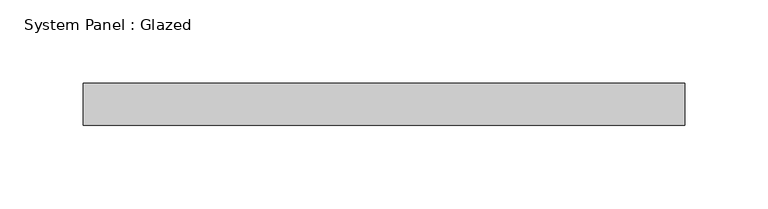
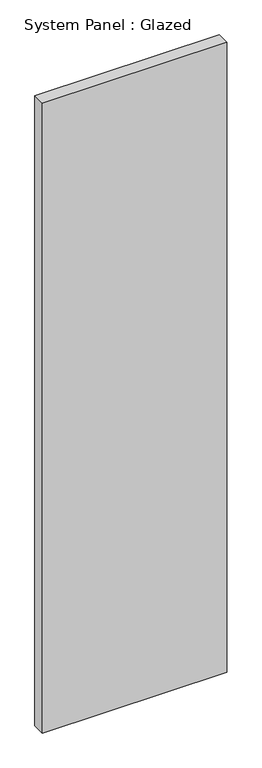
"""IFC4 building model written with IfcOpenShell, lengths in millimetres: plate geometry, System Panel : Glazed."""

from ifc_helpers import new_model, si_unit, origin, origin_with_axes, place, context, project, spatial, polyline, outline, extrude, source, transform, mapped, element, save


def system_panel_glazed_8f314941(model_context):
    return source(origin(), model_context, "Body", "SweptSolid", [
        extrude(outline(polyline([(180.975, 19.05), (-180.975, 19.05), (-180.975, 44.45), (180.975, 44.45), (180.975, 19.05)])), origin_with_axes(), (0.0, 0.0, 1.0), 1308.1),
    ])


if __name__ == "__main__":
    model = new_model("IFC4")
    model_context = context("Model", 3, world=origin())
    ifc_project = project(units=[si_unit("LENGTHUNIT", "METRE", prefix="MILLI")], contexts=[model_context])
    site = spatial("IfcSite", under=ifc_project)
    building = spatial("IfcBuilding", under=site)
    placement = place(None, origin())
    system_panel_glazed_shape = system_panel_glazed_8f314941(model_context)
    element("IfcPlate", 1, ObjectType="System Panel : Glazed", at=placement, inside=building, context=model_context, shape_type="MappedRepresentation", body=[
        mapped(system_panel_glazed_shape, transform((0.0, 0.0, 0.0), x_axis=(1.0, 0.0, 0.0), y_axis=(0.0, 1.0, 0.0), z_axis=(0.0, 0.0, 1.0))),
    ])
    save(model, "model.ifc")

# Revit data of these elements
# Type "System Panel : Glazed"
#   Construction Type Id = "GSP4R"
#   Analytic Construction = "1/8 in Pilkington single glazing"
#   Visual Light Transmittance = 0.9
#   Solar Heat Gain Coefficient = 0.86
#   Heat Transfer Coefficient (U) = 1.18115 BTU/(h·ft²·°F)
#   Define Thermal Properties by = 1
# Element 1 (IfcPlate, "System Panel : Glazed")
#   Materials on its faces: "Glass"
# Materials
#   "Glass": class "Glass", colour RGB 0 128 192, transparency 0.75, Description = "Soda Lime Glass", Cost = 0
